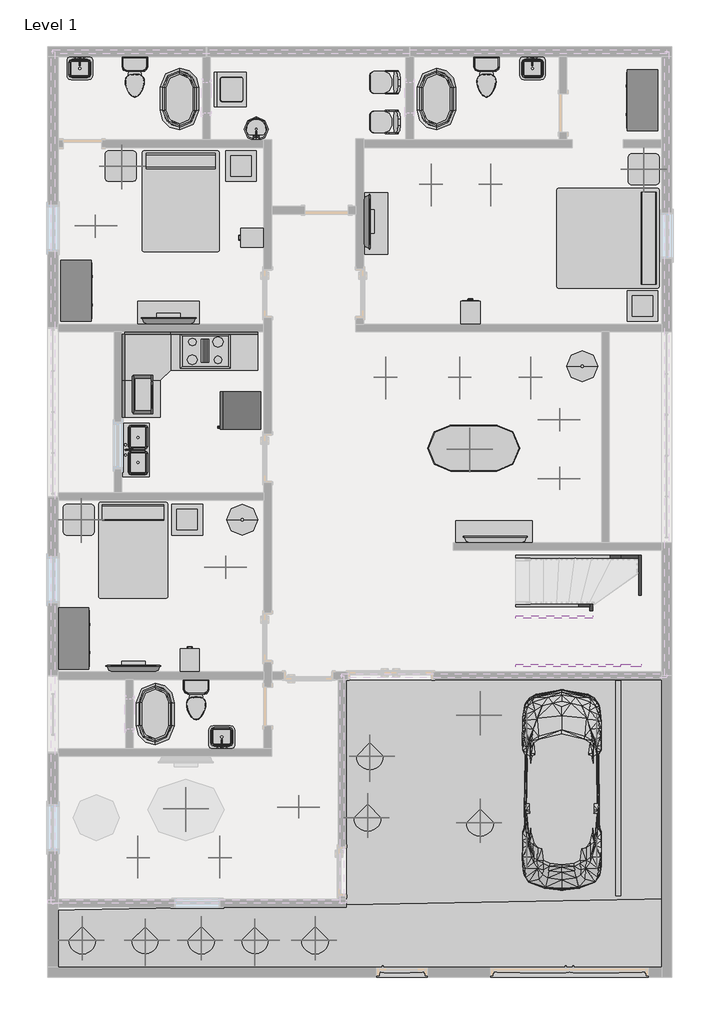
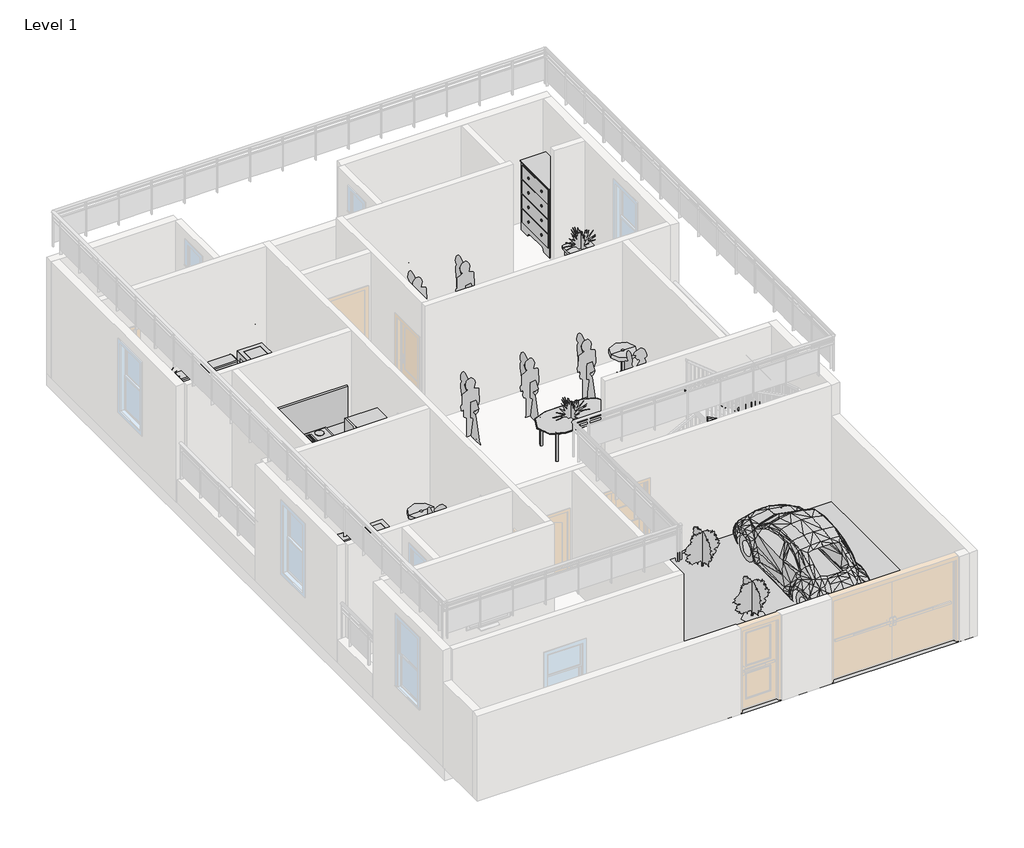
# One storey, part 6 of 6: 28 furniture elements, 20 proxies, 15 flow terminals, 14 geographic elements, 8 members.
"""IFC4 building model written with IfcOpenShell, lengths in millimetres."""

from ifc_helpers import new_model, si_unit, frame, origin, place, context, project, spatial, polyline, outline, extrude, triangles, transform, mapped, element, save
from components import proxy_bb1e6e30, proxy_8a8d5ab2, parking_space_9_x_18_90_deg_fdd9e8f5, rpc_beetle_rpc_beetle_3ce7ba48, rpc_female_69e001fa, proxy_a13a33b2, proxy_718fa39f, flow_terminal_accce45a, flow_terminal_a53be723, flow_terminal_d49f872f, flow_terminal_62a433f7, toilet_domestic_3d_toilet_domestic_3d_f7549cf7, toilet_domestic_3d_toilet_domestic_3d_183bbd19, flow_terminal_04541809, furniture_0253826f, furniture_1fc5af50, furniture_e1791683, furniture_bb55ed6b, furniture_9fa109b2, furniture_3d1d9cbc, furniture_7a3aaa4f, furniture_fdf74506, furniture_b5c51a22, furniture_2c34a4f9, furniture_31d08a24, furniture_c21ab0ed, furniture_87306a90, furniture_1e21b0be, furniture_c625fdf3, rpc_plant_tropical_55f6ff97, rpc_plant_tropical_agave_1_5_93a2a214, rpc_plant_tropical_jungle_flame_3_9c4808c2

model = new_model("IFC4")

# Units and contexts
model_context = context("Model", 3, world=origin())
ifc_project = project(units=[si_unit("LENGTHUNIT", "METRE", prefix="MILLI")], contexts=[model_context])

# Site, building, storey
site = spatial("IfcSite", under=ifc_project)
building = spatial("IfcBuilding", under=site)
storey = spatial("IfcBuildingStorey", under=building, Name="Level 1", Elevation=0.0)

# Proxies
placement = place(None, origin())
element("IfcBuildingElementProxy", 1, Name="Building Element Proxy", at=placement, inside=storey, context=model_context, shape_type="Tessellation", body=[
    triangles([(-14607.1839752, -3299.9680504, 0.0), (-14607.1839752, -4637.9727173, 0.0), (-2211.984169, -4637.9727173, 0.0), (-2211.984169, -3074.4164108, 0.0)], [[1, 2, 3], [3, 4, 1]], closed=False),
])
element("IfcBuildingElementProxy", 2, Name="Building Element Proxy", at=placement, inside=storey, context=model_context, shape_type="Tessellation", body=[
    triangles([(-8688.984169, -3240.9728142, 0.0), (-2211.984169, -3049.3548592, 0.0), (-8841.384169, 1280.2272343, 0.0), (-2211.984169, 1236.1293446, 0.0), (-8638.1843628, 1432.6272343, 0.0), (-2415.1841206, 1280.2272343, 0.0), (-2415.1841206, -3090.3834595, 0.0)], [[3, 1, 5], [5, 1, 7], [7, 2, 4], [4, 6, 7], [7, 6, 5]], closed=False),
])
proxy_shape = proxy_bb1e6e30(model_context)
element("IfcBuildingElementProxy", 3, Name="Cook Top-4 Unit : 36\" x 20\"", ObjectType="Cook Top-4 Unit : 36\" x 20\"", at=placement, inside=storey, context=model_context, shape_type="MappedRepresentation", body=[
    mapped(proxy_shape, transform((-11482.9841185, 7808.0271763, 0.0), x_axis=(1.0, 0.0, 0.0), y_axis=(0.0, 1.0, 0.0), z_axis=(0.0, 0.0, 1.0))),
])
proxy_2_shape = proxy_8a8d5ab2(model_context)
element("IfcBuildingElementProxy", 4, Name="Microwave : 30\" x 16\" x 18\"", ObjectType="Microwave : 30\" x 16\" x 18\"", at=placement, inside=storey, context=model_context, shape_type="MappedRepresentation", body=[
    mapped(proxy_2_shape, transform((-13080.6646243, 6444.1342989, 0.0), x_axis=(0.0, 0.9999999999999999, 0.0), y_axis=(-0.9999999999999999, 0.0, 0.0), z_axis=(0.0, 0.0, 1.0))),
])
parking_space_9_x_18_90_deg_shape = parking_space_9_x_18_90_deg_fdd9e8f5(model_context)
element("IfcBuildingElementProxy", 5, Name="Parking Space : 9' x 18' - 90 deg", ObjectType="Parking Space : 9' x 18' - 90 deg", at=placement, inside=storey, context=model_context, shape_type="MappedRepresentation", body=[
    mapped(parking_space_9_x_18_90_deg_shape, transform((-3278.7841185, -3012.3728237, 0.0), x_axis=(-1.0000000000000004, 0.0, 0.0), y_axis=(0.0, -1.0000000000000004, 0.0), z_axis=(0.0, 0.0, 1.0))),
])
rpc_beetle_rpc_beetle_shape = rpc_beetle_rpc_beetle_3ce7ba48(model_context)
element("IfcBuildingElementProxy", 6, Name="RPC Beetle : RPC Beetle", ObjectType="RPC Beetle : RPC Beetle", at=placement, inside=storey, context=model_context, shape_type="MappedRepresentation", body=[
    mapped(rpc_beetle_rpc_beetle_shape, transform((-4396.3841185, -2148.7728237, 0.0), x_axis=(1.0, 0.0, 0.0), y_axis=(0.0, 1.0, 0.0), z_axis=(0.0, 0.0, 1.0))),
])
rpc_female_shape = rpc_female_69e001fa(model_context)
element("IfcBuildingElementProxy", 7, Name="RPC Female", ObjectType="RPC Female", at=placement, inside=storey, context=model_context, shape_type="MappedRepresentation", body=[
    mapped(rpc_female_shape, transform((-13502.2841185, 10284.5271763, 0.0), x_axis=(0.0, 1.0000000000000002, 0.0), y_axis=(-1.0000000000000002, 0.0, 0.0), z_axis=(0.0, 0.0, 1.0))),
])
element("IfcBuildingElementProxy", 8, Name="RPC Female", ObjectType="RPC Female", at=placement, inside=storey, context=model_context, shape_type="MappedRepresentation", body=[
    mapped(rpc_female_shape, transform((-6996.4115264, 10957.6271763, 0.0), x_axis=(1.0, 0.0, 0.0), y_axis=(0.0, 1.0, 0.0), z_axis=(0.0, 0.0, 1.0))),
])
element("IfcBuildingElementProxy", 9, Name="RPC Female", ObjectType="RPC Female", at=placement, inside=storey, context=model_context, shape_type="MappedRepresentation", body=[
    mapped(rpc_female_shape, transform((-5814.2783903, 10957.6271763, 0.0), x_axis=(1.0, 0.0, 0.0), y_axis=(0.0, 1.0, 0.0), z_axis=(0.0, 0.0, 1.0))),
])
element("IfcBuildingElementProxy", 10, Name="RPC Female", ObjectType="RPC Female", at=placement, inside=storey, context=model_context, shape_type="MappedRepresentation", body=[
    mapped(rpc_female_shape, transform((-6427.2318795, 7122.2271763, 0.0), x_axis=(1.0, 0.0, 0.0), y_axis=(0.0, 1.0, 0.0), z_axis=(0.0, 0.0, 1.0))),
])
element("IfcBuildingElementProxy", 11, Name="RPC Female", ObjectType="RPC Female", at=placement, inside=storey, context=model_context, shape_type="MappedRepresentation", body=[
    mapped(rpc_female_shape, transform((-7900.7506422, 7122.2271763, 0.0), x_axis=(1.0, 0.0, 0.0), y_axis=(0.0, 1.0, 0.0), z_axis=(0.0, 0.0, 1.0))),
])
element("IfcBuildingElementProxy", 12, Name="RPC Female", ObjectType="RPC Female", at=placement, inside=storey, context=model_context, shape_type="MappedRepresentation", body=[
    mapped(rpc_female_shape, transform((-5018.7212974, 7122.2271763, 0.0), x_axis=(1.0, 0.0, 0.0), y_axis=(0.0, 1.0, 0.0), z_axis=(0.0, 0.0, 1.0))),
])
element("IfcBuildingElementProxy", 13, Name="RPC Female", ObjectType="RPC Female", at=placement, inside=storey, context=model_context, shape_type="MappedRepresentation", body=[
    mapped(rpc_female_shape, transform((-4599.5841185, 6441.2059609, 0.0), x_axis=(0.0, -1.0, 0.0), y_axis=(1.0, 0.0, 0.0), z_axis=(0.0, 0.0, 1.0))),
])
element("IfcBuildingElementProxy", 14, Name="RPC Female", ObjectType="RPC Female", at=placement, inside=storey, context=model_context, shape_type="MappedRepresentation", body=[
    mapped(rpc_female_shape, transform((-4599.5841185, 5275.3101398, 0.0), x_axis=(0.0, -1.0, 0.0), y_axis=(1.0, 0.0, 0.0), z_axis=(0.0, 0.0, 1.0))),
])
element("IfcBuildingElementProxy", 15, Name="RPC Female", ObjectType="RPC Female", at=placement, inside=storey, context=model_context, shape_type="MappedRepresentation", body=[
    mapped(rpc_female_shape, transform((-9781.1841185, -1249.3866927, 0.0), x_axis=(0.0, -1.0000000000000004, 0.0), y_axis=(1.0000000000000004, 0.0, 0.0), z_axis=(0.0, 0.0, 1.0))),
])
element("IfcBuildingElementProxy", 16, Name="RPC Female", ObjectType="RPC Female", at=placement, inside=storey, context=model_context, shape_type="MappedRepresentation", body=[
    mapped(rpc_female_shape, transform((-11186.0544122, -2097.9728237, 0.0), x_axis=(-1.0000000000000004, 0.0, 0.0), y_axis=(0.0, -1.0000000000000004, 0.0), z_axis=(0.0, 0.0, 1.0))),
])
element("IfcBuildingElementProxy", 17, Name="RPC Female", ObjectType="RPC Female", at=placement, inside=storey, context=model_context, shape_type="MappedRepresentation", body=[
    mapped(rpc_female_shape, transform((-12811.25893, -2097.9728237, 0.0), x_axis=(-1.0, 0.0, 0.0), y_axis=(0.0, -1.0, 0.0), z_axis=(0.0, 0.0, 1.0))),
])
element("IfcBuildingElementProxy", 18, Name="RPC Female", ObjectType="RPC Female", at=placement, inside=storey, context=model_context, shape_type="MappedRepresentation", body=[
    mapped(rpc_female_shape, transform((-11228.9841185, 3511.6676926, 0.0), x_axis=(0.0, -1.0000000000000004, 0.0), y_axis=(1.0000000000000004, 0.0, 0.0), z_axis=(0.0, 0.0, 1.0))),
])
proxy_3_shape = proxy_a13a33b2(model_context)
element("IfcBuildingElementProxy", 19, Name="Refrigerator : 30\" x 32\" RH", ObjectType="Refrigerator : 30\" x 32\" RH", at=placement, inside=storey, context=model_context, shape_type="MappedRepresentation", body=[
    mapped(proxy_3_shape, transform((-10764.235147, 6622.1646763, 0.0), x_axis=(0.0, -1.0000000000000007, 0.0), y_axis=(1.0000000000000007, 0.0, 0.0), z_axis=(0.0, 0.0, 1.0))),
])
proxy_4_shape = proxy_718fa39f(model_context)
element("IfcBuildingElementProxy", 20, Name="Washer : 27\" x 25\" x 35\"", ObjectType="Washer : 27\" x 25\" x 35\"", at=placement, inside=storey, context=model_context, shape_type="MappedRepresentation", body=[
    mapped(proxy_4_shape, transform((-10708.5345537, 12581.9097078, 0.0), x_axis=(0.0, 1.0000000000000009, 0.0), y_axis=(-1.0000000000000009, 0.0, 0.0), z_axis=(0.0, 0.0, 1.0))),
])

# Flow terminals
flow_terminal_shape = flow_terminal_accce45a(model_context)
element("IfcFlowTerminal", 21, ObjectType="Floor Drain - Round : 5\" Strainer - 2\" Drain", at=placement, inside=storey, context=model_context, shape_type="MappedRepresentation", body=[
    mapped(flow_terminal_shape, transform((-12651.3841185, 12507.0271763, 0.0), x_axis=(1.0, 0.0, 0.0), y_axis=(0.0, 1.0, 0.0), z_axis=(0.0, 0.0, 1.0))),
])
element("IfcFlowTerminal", 22, ObjectType="Floor Drain - Round : 5\" Strainer - 2\" Drain", at=placement, inside=storey, context=model_context, shape_type="MappedRepresentation", body=[
    mapped(flow_terminal_shape, transform((-6275.9841185, 12303.8271763, 0.0), x_axis=(1.0, 0.0, 0.0), y_axis=(0.0, 1.0, 0.0), z_axis=(0.0, 0.0, 1.0))),
])
element("IfcFlowTerminal", 23, ObjectType="Floor Drain - Round : 5\" Strainer - 2\" Drain", at=placement, inside=storey, context=model_context, shape_type="MappedRepresentation", body=[
    mapped(flow_terminal_shape, transform((-10466.9841185, 13446.8271763, 0.0), x_axis=(1.0, 0.0, 0.0), y_axis=(0.0, 1.0, 0.0), z_axis=(0.0, 0.0, 1.0))),
])
element("IfcFlowTerminal", 24, ObjectType="Floor Drain - Round : 5\" Strainer - 2\" Drain", at=placement, inside=storey, context=model_context, shape_type="MappedRepresentation", body=[
    mapped(flow_terminal_shape, transform((-11965.5841185, 86.4271763, 0.0), x_axis=(1.0, 0.0, 0.0), y_axis=(0.0, 1.0, 0.0), z_axis=(0.0, 0.0, 1.0))),
])
flow_terminal_2_shape = flow_terminal_a53be723(model_context)
element("IfcFlowTerminal", 25, ObjectType="Sink Kitchen-Double : 42\" x 21\"", at=placement, inside=storey, context=model_context, shape_type="MappedRepresentation", body=[
    mapped(flow_terminal_2_shape, transform((-12852.2387174, 5823.8379357, 0.0), x_axis=(0.0, 1.0000000000000002, 0.0), y_axis=(-1.0000000000000002, 0.0, 0.0), z_axis=(0.0, 0.0, 1.0))),
])
flow_terminal_3_shape = flow_terminal_d49f872f(model_context)
element("IfcFlowTerminal", 26, ObjectType="Sink Vanity-Round : 19\" x 19\"", at=placement, inside=storey, context=model_context, shape_type="MappedRepresentation", body=[
    mapped(flow_terminal_3_shape, transform((-10370.3323779, 12298.7524416, 0.0), x_axis=(-1.0000000000000004, 0.0, 0.0), y_axis=(0.0, -1.0000000000000004, 0.0), z_axis=(0.0, 0.0, 1.0))),
])
flow_terminal_4_shape = flow_terminal_62a433f7(model_context)
element("IfcFlowTerminal", 27, ObjectType="Sink Vanity-Square : 20\" x 18\"", at=placement, inside=storey, context=model_context, shape_type="MappedRepresentation", body=[
    mapped(flow_terminal_4_shape, transform((-13987.8733591, 13469.8817752, 0.0), x_axis=(1.0, 0.0, 0.0), y_axis=(0.0, 1.0, 0.0), z_axis=(0.0, 0.0, 1.0))),
])
element("IfcFlowTerminal", 28, ObjectType="Sink Vanity-Square : 20\" x 18\"", at=placement, inside=storey, context=model_context, shape_type="MappedRepresentation", body=[
    mapped(flow_terminal_4_shape, transform((-4996.2733591, 13469.8817752, 0.0), x_axis=(1.0, 0.0, 0.0), y_axis=(0.0, 1.0, 0.0), z_axis=(0.0, 0.0, 1.0))),
])
element("IfcFlowTerminal", 29, ObjectType="Sink Vanity-Square : 20\" x 18\"", at=placement, inside=storey, context=model_context, shape_type="MappedRepresentation", body=[
    mapped(flow_terminal_4_shape, transform((-11137.0948779, 88.7725774, 0.0), x_axis=(-1.0000000000000004, 0.0, 0.0), y_axis=(0.0, -1.0000000000000004, 0.0), z_axis=(0.0, 0.0, 1.0))),
])
toilet_domestic_3d_toilet_domestic_3d_shape = toilet_domestic_3d_toilet_domestic_3d_f7549cf7(model_context)
toilet_domestic_3d_toilet_domestic_3d_2_shape = toilet_domestic_3d_toilet_domestic_3d_183bbd19(model_context)
element("IfcFlowTerminal", 30, ObjectType="Toilet-Domestic-3D : Toilet-Domestic-3D", at=placement, inside=storey, context=model_context, shape_type="MappedRepresentation", body=[
    mapped(toilet_domestic_3d_toilet_domestic_3d_shape, transform((-5894.9841185, 13155.3311489, 0.0), x_axis=(1.0, 0.0, 0.0), y_axis=(0.0, 1.0, 0.0), z_axis=(0.0, 0.0, 1.0))),
    mapped(toilet_domestic_3d_toilet_domestic_3d_2_shape, transform((-5894.9841185, 13155.3311489, 0.0), x_axis=(1.0, 0.0, 0.0), y_axis=(0.0, 1.0, 0.0), z_axis=(0.0, 0.0, 1.0))),
])
element("IfcFlowTerminal", 31, ObjectType="Toilet-Domestic-3D : Toilet-Domestic-3D", at=placement, inside=storey, context=model_context, shape_type="MappedRepresentation", body=[
    mapped(toilet_domestic_3d_toilet_domestic_3d_shape, transform((-12879.9841185, 13155.3311489, 0.0), x_axis=(1.0, 0.0, 0.0), y_axis=(0.0, 1.0, 0.0), z_axis=(0.0, 0.0, 1.0))),
    mapped(toilet_domestic_3d_toilet_domestic_3d_2_shape, transform((-12879.9841185, 13155.3311489, 0.0), x_axis=(1.0, 0.0, 0.0), y_axis=(0.0, 1.0, 0.0), z_axis=(0.0, 0.0, 1.0))),
])
element("IfcFlowTerminal", 32, ObjectType="Toilet-Domestic-3D : Toilet-Domestic-3D", at=placement, inside=storey, context=model_context, shape_type="MappedRepresentation", body=[
    mapped(toilet_domestic_3d_toilet_domestic_3d_shape, transform((-11660.7841185, 785.5311489, 0.0), x_axis=(1.0, 0.0, 0.0), y_axis=(0.0, 1.0, 0.0), z_axis=(0.0, 0.0, 1.0))),
    mapped(toilet_domestic_3d_toilet_domestic_3d_2_shape, transform((-11660.7841185, 785.5311489, 0.0), x_axis=(1.0, 0.0, 0.0), y_axis=(0.0, 1.0, 0.0), z_axis=(0.0, 0.0, 1.0))),
])
flow_terminal_5_shape = flow_terminal_04541809(model_context)
element("IfcFlowTerminal", 33, ObjectType="Tub-Free Standing-3D : 30\" x 60\"", at=placement, inside=storey, context=model_context, shape_type="MappedRepresentation", body=[
    mapped(flow_terminal_5_shape, transform((-11990.9841185, 12811.8271763, 0.0), x_axis=(-1.0, 0.0, 0.0), y_axis=(0.0, -1.0, 0.0), z_axis=(0.0, 0.0, 1.0))),
])
element("IfcFlowTerminal", 34, ObjectType="Tub-Free Standing-3D : 30\" x 60\"", at=placement, inside=storey, context=model_context, shape_type="MappedRepresentation", body=[
    mapped(flow_terminal_5_shape, transform((-6885.5841185, 12811.8271763, 0.0), x_axis=(-1.0, 0.0, 0.0), y_axis=(0.0, -1.0, 0.0), z_axis=(0.0, 0.0, 1.0))),
])
element("IfcFlowTerminal", 35, ObjectType="Tub-Free Standing-3D : 30\" x 60\"", at=placement, inside=storey, context=model_context, shape_type="MappedRepresentation", body=[
    mapped(flow_terminal_5_shape, transform((-12473.5841185, 594.4271763, 0.0), x_axis=(1.0000000000000007, 0.0, 0.0), y_axis=(0.0, 1.0000000000000007, 0.0), z_axis=(0.0, 0.0, 1.0))),
])

# Furniture
furniture_shape = furniture_0253826f(model_context)
element("IfcFurniture", 36, ObjectType="Bed-Standard.0001 : Double 54\" x 75\"", at=placement, inside=storey, context=model_context, shape_type="MappedRepresentation", body=[
    mapped(furniture_shape, transform((-13183.2226431, 3891.2222582, 0.0), x_axis=(1.0, 0.0, 0.0), y_axis=(0.0, 1.0, 0.0), z_axis=(0.0, 0.0, 1.0))),
])
furniture_2_shape = furniture_1fc5af50(model_context)
element("IfcFurniture", 37, ObjectType="Bed-Standard.0001 : King 78\" x 80\"", at=placement, inside=storey, context=model_context, shape_type="MappedRepresentation", body=[
    mapped(furniture_2_shape, transform((-3436.3890365, 10314.7157009, 0.0), x_axis=(0.0, -0.9999999999999998, 0.0), y_axis=(0.9999999999999998, 0.0, 0.0), z_axis=(0.0, 0.0, 1.0))),
])
furniture_3_shape = furniture_e1791683(model_context)
element("IfcFurniture", 38, ObjectType="Bed-Standard.0001 : Queen 60\" x 79\"", at=placement, inside=storey, context=model_context, shape_type="MappedRepresentation", body=[
    mapped(furniture_3_shape, transform((-12237.0726431, 10825.4222582, 0.0), x_axis=(1.0, 0.0, 0.0), y_axis=(0.0, 1.0, 0.0), z_axis=(0.0, 0.0, 1.0))),
])
furniture_4_shape = furniture_bb55ed6b(model_context)
element("IfcFurniture", 39, ObjectType="Cabinet-File 2 Drawer : 15\" x 18\"", at=placement, inside=storey, context=model_context, shape_type="MappedRepresentation", body=[
    mapped(furniture_4_shape, transform((-10401.0498184, 9928.0307292, 0.0), x_axis=(0.0, -1.0000000000000002, 0.0), y_axis=(1.0000000000000002, 0.0, 0.0), z_axis=(0.0, 0.0, 1.0))),
])
element("IfcFurniture", 40, ObjectType="Cabinet-File 2 Drawer : 15\" x 18\"", at=placement, inside=storey, context=model_context, shape_type="MappedRepresentation", body=[
    mapped(furniture_4_shape, transform((-6340.3805655, 8427.8928761, 0.0), x_axis=(-0.9999999999999998, 0.0, 0.0), y_axis=(0.0, -0.9999999999999998, 0.0), z_axis=(0.0, 0.0, 1.0))),
])
element("IfcFurniture", 41, ObjectType="Cabinet-File 2 Drawer : 15\" x 18\"", at=placement, inside=storey, context=model_context, shape_type="MappedRepresentation", body=[
    mapped(furniture_4_shape, transform((-11915.6805655, 1519.0928761, 0.0), x_axis=(-1.0000000000000002, 0.0, 0.0), y_axis=(0.0, -1.0000000000000002, 0.0), z_axis=(0.0, 0.0, 1.0))),
])
furniture_5_shape = furniture_9fa109b2(model_context)
element("IfcFurniture", 42, ObjectType="Dresser : 48\" x 72\" x 24\"", at=placement, inside=storey, context=model_context, shape_type="MappedRepresentation", body=[
    mapped(furniture_5_shape, transform((-2433.0211644, 12517.2339164, 0.0), x_axis=(0.0, -1.0000000000000007, 0.0), y_axis=(1.0000000000000007, 0.0, 0.0), z_axis=(0.0, 0.0, 1.0))),
])
element("IfcFurniture", 43, ObjectType="Dresser : 48\" x 72\" x 24\"", at=placement, inside=storey, context=model_context, shape_type="MappedRepresentation", body=[
    mapped(furniture_5_shape, transform((-14411.5470726, 9271.0204361, 0.0), x_axis=(0.0, 1.0, 0.0), y_axis=(-1.0, 0.0, 0.0), z_axis=(0.0, 0.0, 1.0))),
])
element("IfcFurniture", 44, ObjectType="Dresser : 48\" x 72\" x 24\"", at=placement, inside=storey, context=model_context, shape_type="MappedRepresentation", body=[
    mapped(furniture_5_shape, transform((-14462.3470726, 2362.2204361, 0.0), x_axis=(0.0, 1.0000000000000002, 0.0), y_axis=(-1.0000000000000002, 0.0, 0.0), z_axis=(0.0, 0.0, 1.0))),
])
furniture_6_shape = furniture_3d1d9cbc(model_context)
element("IfcFurniture", 45, ObjectType="Seating-Auditorium : 18\" x 24\" x 30\"", at=placement, inside=storey, context=model_context, shape_type="MappedRepresentation", body=[
    mapped(furniture_6_shape, transform((-7711.7087087, 12981.2993074, 0.0), x_axis=(0.0, 1.0000000000000002, 0.0), y_axis=(-1.0000000000000002, 0.0, 0.0), z_axis=(0.0, 0.0, 1.0))),
])
element("IfcFurniture", 46, ObjectType="Seating-Auditorium : 18\" x 24\" x 30\"", at=placement, inside=storey, context=model_context, shape_type="MappedRepresentation", body=[
    mapped(furniture_6_shape, transform((-7711.7087087, 12193.8993074, 0.0), x_axis=(0.0, 1.0000000000000002, 0.0), y_axis=(-1.0000000000000002, 0.0, 0.0), z_axis=(0.0, 0.0, 1.0))),
])
furniture_7_shape = furniture_7a3aaa4f(model_context)
element("IfcFurniture", 47, ObjectType="TV - Flat Screen : 42\"", at=placement, inside=storey, context=model_context, shape_type="MappedRepresentation", body=[
    mapped(furniture_7_shape, transform((-12210.8286326, 8399.9657999, 1041.4), x_axis=(-1.0000000000000004, 0.0, 0.0), y_axis=(0.0, -1.0000000000000004, 0.0), z_axis=(0.0, 0.0, 1.0))),
])
element("IfcFurniture", 48, ObjectType="TV - Flat Screen : 42\"", at=placement, inside=storey, context=model_context, shape_type="MappedRepresentation", body=[
    mapped(furniture_7_shape, transform((-8274.8454949, 10377.3716904, 1041.4), x_axis=(0.0, 1.0000000000000002, 0.0), y_axis=(-1.0000000000000002, 0.0, 0.0), z_axis=(0.0, 0.0, 1.0))),
])
element("IfcFurniture", 49, ObjectType="TV - Flat Screen : 42\"", at=placement, inside=storey, context=model_context, shape_type="MappedRepresentation", body=[
    mapped(furniture_7_shape, transform((-12909.3286326, 1491.1657999, 1041.4), x_axis=(-1.0, 0.0, 0.0), y_axis=(0.0, -1.0, 0.0), z_axis=(0.0, 0.0, 1.0))),
])
furniture_8_shape = furniture_fdf74506(model_context)
element("IfcFurniture", 50, ObjectType="TV - Flat Screen : 50\"", at=placement, inside=storey, context=model_context, shape_type="MappedRepresentation", body=[
    mapped(furniture_8_shape, transform((-5721.1286326, 4056.5657999, 0.0), x_axis=(-1.0000000000000004, 0.0, 0.0), y_axis=(0.0, -1.0000000000000004, 0.0), z_axis=(0.0, 0.0, 1.0))),
])
furniture_9_shape = furniture_b5c51a22(model_context)
element("IfcFurniture", 51, ObjectType="Table-Coffee : 24\" x 24\" x 24\"", at=placement, inside=storey, context=model_context, shape_type="MappedRepresentation", body=[
    mapped(furniture_9_shape, transform((-10790.0498852, 11383.1160985, 0.0), x_axis=(1.0, 0.0, 0.0), y_axis=(0.0, 1.0, 0.0), z_axis=(0.0, 0.0, 1.0))),
])
element("IfcFurniture", 52, ObjectType="Table-Coffee : 24\" x 24\" x 24\"", at=placement, inside=storey, context=model_context, shape_type="MappedRepresentation", body=[
    mapped(furniture_9_shape, transform((-2814.4498852, 8601.8160985, 0.0), x_axis=(1.0, 0.0, 0.0), y_axis=(0.0, 1.0, 0.0), z_axis=(0.0, 0.0, 1.0))),
])
element("IfcFurniture", 53, ObjectType="Table-Coffee : 24\" x 24\" x 24\"", at=placement, inside=storey, context=model_context, shape_type="MappedRepresentation", body=[
    mapped(furniture_9_shape, transform((-11856.8498852, 4360.0160985, 0.0), x_axis=(1.0, 0.0, 0.0), y_axis=(0.0, 1.0, 0.0), z_axis=(0.0, 0.0, 1.0))),
])
furniture_10_shape = furniture_2c34a4f9(model_context)
element("IfcFurniture", 54, ObjectType="Table-Dining Oval : 36\" x 72\"", at=placement, inside=storey, context=model_context, shape_type="MappedRepresentation", body=[
    mapped(furniture_10_shape, transform((-5747.1644464, 6235.7255369, 0.0), x_axis=(1.0, 0.0, 0.0), y_axis=(0.0, 1.0, 0.0), z_axis=(0.0, 0.0, 1.0))),
])
furniture_11_shape = furniture_31d08a24(model_context)
element("IfcFurniture", 55, ObjectType="Table-End : 24\" x 24\"", at=placement, inside=storey, context=model_context, shape_type="MappedRepresentation", body=[
    mapped(furniture_11_shape, transform((-13467.9177488, 11325.9271763, 0.0), x_axis=(1.0, 0.0, 0.0), y_axis=(0.0, 1.0, 0.0), z_axis=(0.0, 0.0, 1.0))),
])
element("IfcFurniture", 56, ObjectType="Table-End : 24\" x 24\"", at=placement, inside=storey, context=model_context, shape_type="MappedRepresentation", body=[
    mapped(furniture_11_shape, transform((-3079.3177488, 11262.4271763, 0.0), x_axis=(1.0, 0.0, 0.0), y_axis=(0.0, 1.0, 0.0), z_axis=(0.0, 0.0, 1.0))),
])
element("IfcFurniture", 57, ObjectType="Table-End : 24\" x 24\"", at=placement, inside=storey, context=model_context, shape_type="MappedRepresentation", body=[
    mapped(furniture_11_shape, transform((-14299.7677488, 4302.8271763, 0.0), x_axis=(1.0, 0.0, 0.0), y_axis=(0.0, 1.0, 0.0), z_axis=(0.0, 0.0, 1.0))),
])
furniture_12_shape = furniture_c21ab0ed(model_context)
element("IfcFurniture", 58, ObjectType="Table-Rectangular : 72\" x 30\"", at=placement, inside=storey, context=model_context, shape_type="MappedRepresentation", body=[
    mapped(furniture_12_shape, transform((-8079.3841185, 10335.3271763, 0.0), x_axis=(0.0, 1.0000000000000002, 0.0), y_axis=(-1.0000000000000002, 0.0, 0.0), z_axis=(0.0, 0.0, 1.0))),
])
element("IfcFurniture", 59, ObjectType="Table-Rectangular : 72\" x 30\"", at=placement, inside=storey, context=model_context, shape_type="MappedRepresentation", body=[
    mapped(furniture_12_shape, transform((-12206.8841185, 8570.0271763, 0.0), x_axis=(1.0, 0.0, 0.0), y_axis=(0.0, 1.0, 0.0), z_axis=(0.0, 0.0, 1.0))),
])
furniture_13_shape = furniture_87306a90(model_context)
element("IfcFurniture", 60, ObjectType="Table-Rectangular : 72\" x 30\" 2", at=placement, inside=storey, context=model_context, shape_type="MappedRepresentation", body=[
    mapped(furniture_13_shape, transform((-5742.5841185, 4208.0271763, 0.0), x_axis=(1.0, 0.0, 0.0), y_axis=(0.0, 1.0, 0.0), z_axis=(0.0, 0.0, 1.0))),
])
furniture_14_shape = furniture_1e21b0be(model_context)
element("IfcFurniture", 61, ObjectType="Table-Round : 36\" Diameter", at=placement, inside=storey, context=model_context, shape_type="MappedRepresentation", body=[
    mapped(furniture_14_shape, transform((-3989.9841185, 7503.2271763, 0.0), x_axis=(1.0, 0.0, 0.0), y_axis=(0.0, 1.0, 0.0), z_axis=(0.0, 0.0, 1.0))),
])
element("IfcFurniture", 62, ObjectType="Table-Round : 36\" Diameter", at=placement, inside=storey, context=model_context, shape_type="MappedRepresentation", body=[
    mapped(furniture_14_shape, transform((-10746.3841185, 4455.2271763, 0.0), x_axis=(1.0, 0.0, 0.0), y_axis=(0.0, 1.0, 0.0), z_axis=(0.0, 0.0, 1.0))),
])
furniture_15_shape = furniture_c625fdf3(model_context)
element("IfcFurniture", 63, ObjectType="Work Station Cubicle : 96\" x 96\"", at=placement, inside=storey, context=model_context, shape_type="MappedRepresentation", body=[
    mapped(furniture_15_shape, transform((-13002.2523663, 8684.0501839, 0.0), x_axis=(1.0, 0.0, 0.0), y_axis=(0.0, 1.0, 0.0), z_axis=(0.0, 0.0, 1.0))),
])

# Geographic elements
rpc_plant_tropical_shape = rpc_plant_tropical_55f6ff97(model_context)
element("IfcGeographicElement", 64, ObjectType="RPC Plant - Tropical", at=placement, inside=storey, context=model_context, shape_type="MappedRepresentation", body=[
    mapped(rpc_plant_tropical_shape, transform((-12676.7841185, -3901.3728237, 0.0), x_axis=(1.0, 0.0, 0.0), y_axis=(0.0, 1.0, 0.0), z_axis=(0.0, 0.0, 1.0))),
])
element("IfcGeographicElement", 65, ObjectType="RPC Plant - Tropical", at=placement, inside=storey, context=model_context, shape_type="MappedRepresentation", body=[
    mapped(rpc_plant_tropical_shape, transform((-10492.3841185, -3901.3728237, 0.0), x_axis=(1.0, 0.0, 0.0), y_axis=(0.0, 1.0, 0.0), z_axis=(0.0, 0.0, 1.0))),
])
element("IfcGeographicElement", 66, ObjectType="RPC Plant - Tropical", at=placement, inside=storey, context=model_context, shape_type="MappedRepresentation", body=[
    mapped(rpc_plant_tropical_shape, transform((-8210.1158104, -243.7728237, 0.0), x_axis=(1.0, 0.0, 0.0), y_axis=(0.0, 1.0, 0.0), z_axis=(0.0, 0.0, 1.0))),
])
rpc_plant_tropical_agave_1_5_shape = rpc_plant_tropical_agave_1_5_93a2a214(model_context)
element("IfcGeographicElement", 67, ObjectType="RPC Plant - Tropical : Agave - 1.5'", at=placement, inside=storey, context=model_context, shape_type="MappedRepresentation", body=[
    mapped(rpc_plant_tropical_agave_1_5_shape, transform((-13133.9841185, 11478.3271763, 609.6), x_axis=(1.0, 0.0, 0.0), y_axis=(0.0, 1.0, 0.0), z_axis=(0.0, 0.0, 1.0))),
])
element("IfcGeographicElement", 68, ObjectType="RPC Plant - Tropical : Agave - 1.5'", at=placement, inside=storey, context=model_context, shape_type="MappedRepresentation", body=[
    mapped(rpc_plant_tropical_agave_1_5_shape, transform((-2770.7841185, 11414.8271763, 609.6), x_axis=(1.0, 0.0, 0.0), y_axis=(0.0, 1.0, 0.0), z_axis=(0.0, 0.0, 1.0))),
])
element("IfcGeographicElement", 69, ObjectType="RPC Plant - Tropical : Agave - 1.5'", at=placement, inside=storey, context=model_context, shape_type="MappedRepresentation", body=[
    mapped(rpc_plant_tropical_agave_1_5_shape, transform((-6225.1841185, 5852.2271763, 736.6), x_axis=(1.0, 0.0, 0.0), y_axis=(0.0, 1.0, 0.0), z_axis=(0.0, 0.0, 1.0))),
])
element("IfcGeographicElement", 70, ObjectType="RPC Plant - Tropical : Agave - 1.5'", at=placement, inside=storey, context=model_context, shape_type="MappedRepresentation", body=[
    mapped(rpc_plant_tropical_agave_1_5_shape, transform((-13940.4341185, 4455.2271763, 609.6), x_axis=(1.0, 0.0, 0.0), y_axis=(0.0, 1.0, 0.0), z_axis=(0.0, 0.0, 1.0))),
])
element("IfcGeographicElement", 71, ObjectType="RPC Plant - Tropical : Agave - 1.5'", at=placement, inside=storey, context=model_context, shape_type="MappedRepresentation", body=[
    mapped(rpc_plant_tropical_agave_1_5_shape, transform((-11863.9841185, -1285.1728237, 736.6), x_axis=(1.0, 0.0, 0.0), y_axis=(0.0, 1.0, 0.0), z_axis=(0.0, 0.0, 1.0))),
])
rpc_plant_tropical_jungle_flame_3_shape = rpc_plant_tropical_jungle_flame_3_9c4808c2(model_context)
element("IfcGeographicElement", 72, ObjectType="RPC Plant - Tropical : Jungle Flame - 3'", at=placement, inside=storey, context=model_context, shape_type="MappedRepresentation", body=[
    mapped(rpc_plant_tropical_jungle_flame_3_shape, transform((-13921.3841185, -3901.3728237, 0.0), x_axis=(1.0, 0.0, 0.0), y_axis=(0.0, 1.0, 0.0), z_axis=(0.0, 0.0, 1.0))),
])
element("IfcGeographicElement", 73, ObjectType="RPC Plant - Tropical : Jungle Flame - 3'", at=placement, inside=storey, context=model_context, shape_type="MappedRepresentation", body=[
    mapped(rpc_plant_tropical_jungle_flame_3_shape, transform((-9298.5841185, -3901.3728237, 0.0), x_axis=(1.0, 0.0, 0.0), y_axis=(0.0, 1.0, 0.0), z_axis=(0.0, 0.0, 1.0))),
])
element("IfcGeographicElement", 74, ObjectType="RPC Plant - Tropical : Jungle Flame - 3'", at=placement, inside=storey, context=model_context, shape_type="MappedRepresentation", body=[
    mapped(rpc_plant_tropical_jungle_flame_3_shape, transform((-11559.1841185, -3901.3728237, 0.0), x_axis=(1.0, 0.0, 0.0), y_axis=(0.0, 1.0, 0.0), z_axis=(0.0, 0.0, 1.0))),
])
element("IfcGeographicElement", 75, ObjectType="RPC Plant - Tropical : Jungle Flame - 3'", at=placement, inside=storey, context=model_context, shape_type="MappedRepresentation", body=[
    mapped(rpc_plant_tropical_jungle_flame_3_shape, transform((-6021.9841185, 569.0271763, 0.0), x_axis=(1.0, 0.0, 0.0), y_axis=(0.0, 1.0, 0.0), z_axis=(0.0, 0.0, 1.0))),
])
element("IfcGeographicElement", 76, ObjectType="RPC Plant - Tropical : Jungle Flame - 3'", at=placement, inside=storey, context=model_context, shape_type="MappedRepresentation", body=[
    mapped(rpc_plant_tropical_jungle_flame_3_shape, transform((-6021.9841185, -1564.5728237, 0.0), x_axis=(1.0, 0.0, 0.0), y_axis=(0.0, 1.0, 0.0), z_axis=(0.0, 0.0, 1.0))),
])
element("IfcGeographicElement", 77, ObjectType="RPC Plant - Tropical : Jungle Flame - 3'", at=placement, inside=storey, context=model_context, shape_type="MappedRepresentation", body=[
    mapped(rpc_plant_tropical_jungle_flame_3_shape, transform((-8257.1841185, -1462.9728237, 0.0), x_axis=(1.0, 0.0, 0.0), y_axis=(0.0, 1.0, 0.0), z_axis=(0.0, 0.0, 1.0))),
])

# Members
element("IfcMember", 78, ObjectType="Stringer - 2\" Width", at=placement, inside=storey, context=model_context, shape_type="SweptSolid", body=[
    extrude(outline(polyline([(229.639954, -5314.5158104), (0.0, -5314.5158104), (0.0, -5094.7534928), (962.500629, -3227.0986187), (1305.3956453, -3227.0986187), (229.639954, -5314.5158104)])), frame((0.0, 3693.2271763, 0.0), z_axis=(0.0, 1.0, 0.0), x_axis=(0.0, 0.0, 1.0)), (0.0, 0.0, 1.0), 50.8),
])
element("IfcMember", 79, ObjectType="Stringer - 2\" Width", at=placement, inside=storey, context=model_context, shape_type="SweptSolid", body=[
    extrude(outline(polyline([(-3227.0986187, 3693.2271763), (-3227.0986187, 3744.0271763), (-2872.3841185, 3744.0271763), (-2872.3841185, 3693.2271763), (-3227.0986187, 3693.2271763)])), frame((0.0, 0.0, 962.500629), z_axis=(0.0, 0.0, 1.0), x_axis=(1.0, 0.0, 0.0)), (0.0, 0.0, 1.0), 342.8950162),
])
element("IfcMember", 80, ObjectType="Stringer - 2\" Width", at=placement, inside=storey, context=model_context, shape_type="SweptSolid", body=[
    extrude(outline(polyline([(3744.0271763, 1289.0952212), (3744.0271763, 1000.5956453), (3574.5046933, 1000.5956453), (1585.0271763, 1638.9682298), (1585.0271763, 1969.9972697), (1622.0072936, 1969.9972697), (3744.0271763, 1289.0952212)])), frame((-2872.3841185, 0.0, 0.0), z_axis=(1.0, 0.0, 0.0), x_axis=(0.0, 1.0, 0.0)), (0.0, 0.0, 1.0), 50.8),
])
element("IfcMember", 81, ObjectType="Stringer - 2\" Width", at=placement, inside=storey, context=model_context, shape_type="SweptSolid", body=[
    extrude(outline(polyline([(-2821.5841185, 1585.0271763), (-2821.5841185, 1534.2271763), (-3227.0986187, 1534.2271763), (-3227.0986187, 1585.0271763), (-2821.5841185, 1585.0271763)])), frame((0.0, 0.0, 1649.8904473), z_axis=(0.0, 0.0, 1.0), x_axis=(1.0, 0.0, 0.0)), (0.0, 0.0, 1.0), 320.1068224),
])
element("IfcMember", 82, ObjectType="Stringer - 2\" Width", at=placement, inside=storey, context=model_context, shape_type="SweptSolid", body=[
    extrude(outline(polyline([(1649.8904473, -3227.0986187), (1969.9972697, -3227.0986187), (3045.7529609, -5314.5158104), (2725.6461385, -5314.5158104), (1649.8904473, -3227.0986187)])), frame((0.0, 1534.2271763, 0.0), z_axis=(0.0, 1.0, 0.0), x_axis=(0.0, 0.0, 1.0)), (0.0, 0.0, 1.0), 50.8),
])
element("IfcMember", 83, ObjectType="Stringer - 2\" Width", at=placement, inside=storey, context=model_context, shape_type="SweptSolid", body=[
    extrude(outline(polyline([(176.1764461, -5314.5158104), (0.0, -5314.5158104), (0.0, -5048.2541658), (987.1410923, -3837.5841185), (1380.418648, -3837.5841185), (176.1764461, -5314.5158104)])), frame((0.0, 2728.0271763, 0.0), z_axis=(0.0, 1.0, 0.0), x_axis=(0.0, 0.0, 1.0)), (0.0, 0.0, 1.0), 50.8),
])
element("IfcMember", 84, ObjectType="Stringer - 2\" Width", at=placement, inside=storey, context=model_context, shape_type="SweptSolid", body=[
    extrude(outline(polyline([(2778.8271763, 1573.2682978), (2778.8271763, 1028.5617647), (2744.5849589, 1028.5617647), (2550.2271763, 1360.465107), (2550.2271763, 1926.1409689), (2572.1900588, 1926.1409689), (2778.8271763, 1573.2682978)])), frame((-3837.5841185, 0.0, 0.0), z_axis=(1.0, 0.0, 0.0), x_axis=(0.0, 1.0, 0.0)), (0.0, 0.0, 1.0), 50.8),
])
element("IfcMember", 85, ObjectType="Stringer - 2\" Width", at=placement, inside=storey, context=model_context, shape_type="SweptSolid", body=[
    extrude(outline(polyline([(1532.8634131, -3786.7841185), (1926.1409689, -3786.7841185), (3171.8038432, -5314.5158104), (2778.5262875, -5314.5158104), (1532.8634131, -3786.7841185)])), frame((0.0, 2499.4271763, 0.0), z_axis=(0.0, 1.0, 0.0), x_axis=(0.0, 0.0, 1.0)), (0.0, 0.0, 1.0), 50.8),
])

save(model, "model.ifc")

# Revit data of these elements
# Type "Cook Top-4 Unit : 36\" x 20\""
#   Assembly Code = "E1090400"
#   Depth = 2' - 0"
#   Width = 3' - 0"
#   Burner Material = Steel, Chrome Plated
#   Cooktop Material = Steel, Polished
#   Default Elevation = 0
# Type "Microwave : 30\" x 16\" x 18\""
#   Assembly Code = "E1090400"
#   Depth = 1' - 4"
#   Height = 1' - 6"
#   Width = 2' - 6"
#   Microwave Material = Laminate, Linen, Matte
#   Default Elevation = 0
# Type "Parking Space : 9' x 18' - 90 deg"
#   Angle = 90.00°
#   Parking Length = 18' - 0"
#   Parking Width = 9' - 0"
#   pl = 14' - 0"
#   pw = 7' - 0"
# Type "RPC Beetle : RPC Beetle"
#   built-in parameter 1005195 = "RPC-16-0U6E-L4EG-ENH1-J3KF-SVEL-0TX4-C0"
#   Height = 0
# Type "RPC Female"
#   built-in parameter 1005195 = "RPC-8-FXA2-QQQ0-UGV2-6"
#   Height = 0
# Type "Refrigerator : 30\" x 32\" RH"
#   Label = "REF."
#   Assembly Code = "E1090400"
#   Depth = 2' - 7 3/4"
#   Handle = 2' - 3"
#   Height = 5' - 10"
#   Rear Clearance = 0' - 2"
#   Top Door Height = 1' - 8"
#   Width = 2' - 5 3/8"
#   Material = Carpet (1)
#   Default Elevation = 0
# Type "Washer : 27\" x 25\" x 35\""
#   Label = "W"
#   Assembly Code = "E1090400"
#   Depth = 2' - 1"
#   Height = 2' - 11"
#   Width = 2' - 3"
#   Washer Material = Steel, Paint Finish, Ivory, Matte
#   Default Elevation = 0
# Type "Floor Drain - Round : 5\" Strainer - 2\" Drain"
#   WFU = 2
#   Strainer Height = 0' - 3 1/4"
#   Strainer Radius = 0' - 2 1/2"
#   Strainer Diameter = 0' - 5"
#   Radius 6 = 0' - 0 5/8"
#   Radius 5 = 0' - 1 1/4"
#   Radius 4 = 0' - 1 7/8"
#   Radius 2 = 0' - 3.04167"
#   Radius 1 = 0' - 2.02083"
#   Radius 3 = 0' - 2 1/32"
#   Pipe Radius = 1"
#   Pipe Diameter = 2"
#   Height 2 = 0' - 0.725"
#   Height 1 = 0' - 1 13/16"
#   Body Radius = 0' - 4 1/16"
#   Body Height = 0' - 3 5/8"
#   Body Diameter = 0' - 8 1/8"
#   Drain Material = none
#   HWFU = 0
#   Default Elevation = 0
#   CWFU = 0
# Type "Sink Kitchen-Double : 42\" x 21\""
#   Assembly Code = "D2010410"
#   Counter Height = 3' - 0"
#   Depth = 1' - 9"
#   Width = 3' - 6"
#   Faucet Material = Steel, Polished
#   Sink Material = Steel, Polished
#   Default Elevation = 0
# Type "Sink Vanity-Round : 19\" x 19\""
#   Assembly Code = "D2010400"
#   Top Of Counter = 2' - 7"
#   Basin Material = Porcelain, Linen
#   Faucet Material = Steel, Polished
#   Default Elevation = 0
# Type "Sink Vanity-Square : 20\" x 18\""
#   Assembly Code = "D2010400"
#   Counter Height = 2' - 7"
#   Depth = 1' - 6"
#   Width = 1' - 8"
#   Basin Material = Porcelain, Linen
#   Faucet Material = Steel, Polished
#   Default Elevation = 0
# Type "Toilet-Domestic-3D : Toilet-Domestic-3D"
#   Assembly Code = "D2010110"
#   Toilet - Bowl/Basin Material = Porcelain, Linen
#   Toilet - Seat Material = Laminate, Linen, Matte
#   Default Elevation = 0
# Type "Tub-Free Standing-3D : 30\" x 60\""
#   Assembly Code = "D2010110"
#   Height = 1' - 6"
#   Length = 4' - 0"
#   Width = 2' - 6"
#   Tub Material = Porcelain, Ivory
#   Default Elevation = 0
# Type "Bed-Standard.0001 : Double 54\" x 75\""
#   Assembly Code = "E2020200"
#   Length = 6' - 3"
#   Width = 4' - 6"
#   Leg Material = Steel, Chrome Plated
#   Mattress Material = Pine
#   Default Elevation = 0
# Type "Bed-Standard.0001 : King 78\" x 80\""
#   Assembly Code = "E2020200"
#   Length = 6' - 8"
#   Width = 6' - 6"
#   Leg Material = Steel, Chrome Plated
#   Mattress Material = Softwood, Lumber
#   Default Elevation = 0
# Type "Bed-Standard.0001 : Queen 60\" x 79\""
#   Assembly Code = "E2020200"
#   Length = 6' - 7"
#   Width = 5' - 0"
#   Leg Material = Steel, Chrome Plated
#   Mattress Material = Pine
#   Default Elevation = 0
# Type "Cabinet-File 2 Drawer : 15\" x 18\""
#   Assembly Code = "E2020200"
#   Depth = 1' - 6"
#   Height = 2' - 5"
#   Width = 1' - 3"
#   Cabinet Material = Steel, Paint Finish, Ivory, Glossy
#   Handle Material = Steel, Chrome Plated
#   Default Elevation = 0
# Type "Dresser : 48\" x 72\" x 24\""
#   Assembly Code = "E2020200"
#   Depth = 2' - 0"
#   Height = 6' - 0"
#   Width = 4' - 0"
#   Dresser Material = Wood Door Panel - Birch
#   Drawer Material = Wood Door Panel - Birch
#   Knob Material = Cherry
#   Default Elevation = 0
# Type "Seating-Auditorium : 18\" x 24\" x 30\""
#   Assembly Code = "E2020200"
#   Seat Material = Linen, Beige
#   Frame Material = Steel, Paint Finish, Dark Gray, Matte
#   Default Elevation = 0
# Type "TV - Flat Screen : 42\""
#   SinAng = 0' - 0.0193"
#   L = 3' - 0.71517"
#   H = 1' - 8.65418"
#   Thickness = 0' - 4.33071"
#   Diagonal = 3' - 6.12598"
#   CosAng = 0' - 0.03431"
#   Stand [instance default] = yes
#   Default Elevation = 0
# Type "TV - Flat Screen : 50\""
#   SinAng = 0' - 0.0193"
#   L = 3' - 7.57782"
#   H = 2' - 0.51477"
#   Thickness = 0' - 4.33071"
#   Diagonal = 4' - 2"
#   CosAng = 0' - 0.03431"
#   Stand [instance default] = yes
#   Default Elevation = 0
# Type "Table-Coffee : 24\" x 24\" x 24\""
#   Assembly Code = "E2020200"
#   Height = 2' - 0"
#   Length = 2' - 0"
#   Width = 2' - 0"
#   Top Material = none
#   Frame Material = none
#   Default Elevation = 0
# Type "Table-Dining Oval : 36\" x 72\""
#   Assembly Code = "E2020200"
#   Length = 6' - 0"
#   Width = 3' - 0"
#   Base Material = Steel, Chrome Plated
#   Top Material = Glass - Clear, Grey
#   Default Elevation = 0
#   Description = (empty or 0)
# Type "Table-End : 24\" x 24\""
#   Assembly Code = "E2020200"
#   Height = 2' - 0"
#   Length = 2' - 0"
#   Width = 2' - 0"
#   Base Material = Birch
#   Top Material = Laminate, Ivory, Matte
#   Default Elevation = 0
# Type "Table-Rectangular : 72\" x 30\""
#   Assembly Code = "E2020200"
#   Height = 2' - 0"
#   Length = 4' - 0"
#   Width = 1' - 6"
#   Base Material = Birch
#   Top Material = Birch
#   Default Elevation = 0
# Type "Table-Rectangular : 72\" x 30\" 2"
#   Assembly Code = "E2020200"
#   Height = 2' - 0"
#   Length = 5' - 0"
#   Width = 1' - 6"
#   Base Material = Birch
#   Top Material = Birch
#   Default Elevation = 0
# Type "Table-Round : 36\" Diameter"
#   Assembly Code = "E2020200"
#   Base Radius = 0' - 10"
#   Height = 2' - 2"
#   Radius = 1' - 0"
#   Base Material = Steel, Chrome Plated
#   Top Material = Birch
#   Default Elevation = 0
# Type "Work Station Cubicle : 96\" x 96\""
#   Assembly Code = "E2020"
#   Desktop Height = 2' - 6"
#   Desktop1 Width = 2' - 4"
#   Desktop2 Width = 2' - 4"
#   Panel Height = 5' - 6"
#   Panel1 Length = 2' - 5"
#   Panel2 Length = 5' - 8"
#   Cube Panel Material = Textile - Light Gray
#   Work Top Material = Laminate, Ivory, Matte
#   Default Elevation = 0
# Type "RPC Plant - Tropical"
#   built-in parameter 1005198 = "{2, 15},{39, RPC-16-FWM5-GM7X-C67P-4000-ST1L-LVER-AU},{1, 0},{1, 0},{2, 13},{1, 8},{5, Color},{1, 0},{1, 0},{3, 0.8},{3, 0.8},{3, 0.8},{1, 8},{7, BBoxMin},{1, 0},{1, 0},{1, 0},{1, 0},{1, 0},{1, 8},{7, BBoxMax},{1, 0},{1, 0},{1, 0},{1, 0},{1, 0},{2, 11},{9, RPCTypeId},{1, 0},{1, 0},{39, RPC-16-FWM5-GM7X-C67P-4000-ST1L-LVER-AU},{1, 6},{14, RPCPlantHeight},{1, 0},{1, 0},{1, 3},{2, 11},{7, keyword},{1, 0},{1, 0},{35, :RPCs:Shrubs [General]:Geometry:RPC},{2, 11},{8, category},{1, 0},{1, 0},{16, Shrubs [General]},{2, 11},{12, LocalizedUID},{1, 0},{1, 0},{10, Crane Lily},{2, 14},{6, Height},{1, 0},{1, 0},{1, 3},{1, 2},{16, Cast Reflections},{1, 0},{1, 0},{1, 0},{1, 2},{12, Cast Shadows},{1, 0},{1, 0},{1, 1},{1, 2},{9, Lock View},{1, 0},{1, 0},{1, 0},{1, 4},{5, ViewC},{1, 0},{1, 0},{1, 0},{21, assetlibrary_base.fbx},{1, 5},"
#   built-in parameter 1005195 = "RPC-16-FWM5-GM7X-C67P-4000-ST1L-LVER-AU"
#   Assembly Code = "G2050500"
#   Height = 3' - 0"
#   Default Elevation = 0
# Type "RPC Plant - Tropical : Agave - 1.5'"
#   built-in parameter 1005198 = "{2, 15},{39, RPC-16-G1GJ-63FX-7K5P-N000-ST1L-LVER-AU},{1, 0},{1, 0},{2, 13},{1, 8},{5, Color},{1, 0},{1, 0},{3, 0.8},{3, 0.8},{3, 0.8},{1, 8},{7, BBoxMin},{1, 0},{1, 0},{1, 0},{1, 0},{1, 0},{1, 8},{7, BBoxMax},{1, 0},{1, 0},{1, 0},{1, 0},{1, 0},{2, 11},{9, RPCTypeId},{1, 0},{1, 0},{39, RPC-16-G1GJ-63FX-7K5P-N000-ST1L-LVER-AU},{1, 6},{14, RPCPlantHeight},{1, 0},{1, 0},{3, 1.5},{2, 11},{7, keyword},{1, 0},{1, 0},{35, :RPCs:Plants [General]:Geometry:RPC},{2, 11},{8, category},{1, 0},{1, 0},{16, Plants [General]},{2, 11},{12, LocalizedUID},{1, 0},{1, 0},{5, Agave},{2, 14},{6, Height},{1, 0},{1, 0},{3, 1.5},{1, 2},{16, Cast Reflections},{1, 0},{1, 0},{1, 0},{1, 2},{12, Cast Shadows},{1, 0},{1, 0},{1, 1},{1, 2},{9, Lock View},{1, 0},{1, 0},{1, 0},{1, 4},{5, ViewC},{1, 0},{1, 0},{1, 0},{21, assetlibrary_base.fbx},{1, 5},"
#   built-in parameter 1005195 = "RPC-16-G1GJ-63FX-7K5P-N000-ST1L-LVER-AU"
#   Type Comments = "Agave"
#   Assembly Code = "G2050500"
#   Height = 1' - 6"
#   Default Elevation = 0
# Type "RPC Plant - Tropical : Jungle Flame - 3'"
#   built-in parameter 1005198 = "{2, 15},{39, RPC-16-FUVJ-JWG0-MWGK-8000-ST1L-LVER-AU},{1, 0},{1, 0},{2, 13},{1, 8},{5, Color},{1, 0},{1, 0},{3, 0.8},{3, 0.8},{3, 0.8},{1, 8},{7, BBoxMin},{1, 0},{1, 0},{1, 0},{1, 0},{1, 0},{1, 8},{7, BBoxMax},{1, 0},{1, 0},{1, 0},{1, 0},{1, 0},{2, 11},{9, RPCTypeId},{1, 0},{1, 0},{39, RPC-16-FUVJ-JWG0-MWGK-8000-ST1L-LVER-AU},{1, 6},{14, RPCPlantHeight},{1, 0},{1, 0},{1, 3},{2, 11},{7, keyword},{1, 0},{1, 0},{35, :RPCs:Shrubs [General]:Geometry:RPC},{2, 11},{8, category},{1, 0},{1, 0},{16, Shrubs [General]},{2, 11},{12, LocalizedUID},{1, 0},{1, 0},{12, Jungle Flame},{2, 14},{6, Height},{1, 0},{1, 0},{1, 3},{1, 2},{16, Cast Reflections},{1, 0},{1, 0},{1, 0},{1, 2},{12, Cast Shadows},{1, 0},{1, 0},{1, 1},{1, 2},{9, Lock View},{1, 0},{1, 0},{1, 0},{1, 4},{5, ViewC},{1, 0},{1, 0},{1, 0},{21, assetlibrary_base.fbx},{1, 5},"
#   built-in parameter 1005195 = "RPC-16-FUVJ-JWG0-MWGK-8000-ST1L-LVER-AU"
#   Type Comments = "Jungle Flame"
#   Assembly Code = "G2050500"
#   Height = 3' - 0"
#   Default Elevation = 0
# Elements 1, 2 (IfcBuildingElementProxy)
#   Material = Plant
#   Phase Created = New Construction
# Element 3 (IfcBuildingElementProxy, "Cook Top-4 Unit : 36\" x 20\"")
#   Phase Created = New Construction
#   Materials on its faces: "Steel, Chrome Plated", "Steel, Polished"
# Element 4 (IfcBuildingElementProxy, "Microwave : 30\" x 16\" x 18\"")
#   Phase Created = New Construction
#   Materials on its faces: "Laminate, Linen, Matte", "Glass"
# Element 5 (IfcBuildingElementProxy, "Parking Space : 9' x 18' - 90 deg")
#   Phase Created = New Construction
#   Materials on its faces: "Parking Stripe"
# Element 6 (IfcBuildingElementProxy, "RPC Beetle : RPC Beetle")
#   Phase Created = New Construction
# Elements 7, 8, 9, 10, 11, 12, 13, 14, 15, 16, 17, 18 (IfcBuildingElementProxy, "RPC Female")
#   Phase Created = New Construction
# Element 19 (IfcBuildingElementProxy, "Refrigerator : 30\" x 32\" RH")
#   Phase Created = New Construction
#   Materials on its faces: "Carpet (1)", "Steel, Chrome Plated"
# Element 20 (IfcBuildingElementProxy, "Washer : 27\" x 25\" x 35\"")
#   Phase Created = New Construction
#   Materials on its faces: "Steel, Paint Finish, Ivory, Matte"
# Element 21 (IfcFlowTerminal, "Floor Drain - Round : 5\" Strainer - 2\" Drain")
#   Mark = "4"
#   Phase Created = New Construction
# Element 22 (IfcFlowTerminal, "Floor Drain - Round : 5\" Strainer - 2\" Drain")
#   Mark = "8"
#   Phase Created = New Construction
# Element 23 (IfcFlowTerminal, "Floor Drain - Round : 5\" Strainer - 2\" Drain")
#   Mark = "9"
#   Phase Created = New Construction
# Element 24 (IfcFlowTerminal, "Floor Drain - Round : 5\" Strainer - 2\" Drain")
#   Mark = "16"
#   Phase Created = New Construction
# Element 25 (IfcFlowTerminal, "Sink Kitchen-Double : 42\" x 21\"")
#   Mark = "12"
#   Phase Created = New Construction
#   Materials on its faces: "Steel, Polished"
# Element 26 (IfcFlowTerminal, "Sink Vanity-Round : 19\" x 19\"")
#   Mark = "10"
#   Phase Created = New Construction
#   Materials on its faces: "Porcelain, Linen", "Steel, Polished"
# Element 27 (IfcFlowTerminal, "Sink Vanity-Square : 20\" x 18\"")
#   Mark = "2"
#   Phase Created = New Construction
#   Materials on its faces: "Porcelain, Linen", "Steel, Polished"
# Element 28 (IfcFlowTerminal, "Sink Vanity-Square : 20\" x 18\"")
#   Mark = "7"
#   Phase Created = New Construction
#   Materials on its faces: "Porcelain, Linen", "Steel, Polished"
# Element 29 (IfcFlowTerminal, "Sink Vanity-Square : 20\" x 18\"")
#   Mark = "14"
#   Phase Created = New Construction
#   Materials on its faces: "Porcelain, Linen", "Steel, Polished"
# Element 30 (IfcFlowTerminal, "Toilet-Domestic-3D : Toilet-Domestic-3D")
#   Mark = "6"
#   Phase Created = New Construction
#   Materials on its faces: "Porcelain, Linen", "Laminate, Linen, Matte"
# Element 31 (IfcFlowTerminal, "Toilet-Domestic-3D : Toilet-Domestic-3D")
#   Mark = "11"
#   Phase Created = New Construction
#   Materials on its faces: "Porcelain, Linen", "Laminate, Linen, Matte"
# Element 32 (IfcFlowTerminal, "Toilet-Domestic-3D : Toilet-Domestic-3D")
#   Mark = "15"
#   Phase Created = New Construction
#   Materials on its faces: "Porcelain, Linen", "Laminate, Linen, Matte"
# Element 33 (IfcFlowTerminal, "Tub-Free Standing-3D : 30\" x 60\"")
#   Mark = "1"
#   Phase Created = New Construction
#   Materials on its faces: "Porcelain, Ivory"
# Element 34 (IfcFlowTerminal, "Tub-Free Standing-3D : 30\" x 60\"")
#   Mark = "5"
#   Phase Created = New Construction
#   Materials on its faces: "Porcelain, Ivory"
# Element 35 (IfcFlowTerminal, "Tub-Free Standing-3D : 30\" x 60\"")
#   Mark = "13"
#   Phase Created = New Construction
#   Materials on its faces: "Porcelain, Ivory"
# Element 36 (IfcFurniture, "Bed-Standard.0001 : Double 54\" x 75\"")
#   Phase Created = New Construction
#   Materials on its faces: "Linen, White", "Steel, Chrome Plated"
# Element 37 (IfcFurniture, "Bed-Standard.0001 : King 78\" x 80\"")
#   Phase Created = New Construction
#   Materials on its faces: "Linen, White", "Steel, Chrome Plated"
# Element 38 (IfcFurniture, "Bed-Standard.0001 : Queen 60\" x 79\"")
#   Phase Created = New Construction
#   Materials on its faces: "Linen, White", "Steel, Chrome Plated"
# Elements 39, 40, 41 (IfcFurniture, "Cabinet-File 2 Drawer : 15\" x 18\"")
#   Phase Created = New Construction
#   Materials on its faces: "Steel, Chrome Plated", "Steel, Paint Finish, Ivory, Glossy"
# Elements 42, 43, 44 (IfcFurniture, "Dresser : 48\" x 72\" x 24\"")
#   Phase Created = New Construction
#   Materials on its faces: "Laminate, Ivory, Matte", "Cherry", "Wood Door Panel - Birch"
# Elements 45, 46 (IfcFurniture, "Seating-Auditorium : 18\" x 24\" x 30\"")
#   Phase Created = New Construction
#   Materials on its faces: "Steel, Paint Finish, Dark Gray, Matte", "Linen, Beige"
# Elements 47, 48, 49 (IfcFurniture, "TV - Flat Screen : 42\"")
#   Stand = yes
#   Phase Created = New Construction
#   Materials on its faces: "TV - Black", "TV - Glass", "TV - Screen"
# Element 50 (IfcFurniture, "TV - Flat Screen : 50\"")
#   Stand = yes
#   Phase Created = New Construction
#   Materials on its faces: "TV - Black", "TV - Glass", "TV - Screen"
# Elements 51, 52, 53 (IfcFurniture, "Table-Coffee : 24\" x 24\" x 24\"")
#   Phase Created = New Construction
#   Materials on its faces: "Glass - Clear, Grey"
# Element 54 (IfcFurniture, "Table-Dining Oval : 36\" x 72\"")
#   Phase Created = New Construction
#   Materials on its faces: "Steel, Chrome Plated", "Glass - Clear, Grey"
# Elements 55, 56, 57 (IfcFurniture, "Table-End : 24\" x 24\"")
#   Phase Created = New Construction
#   Materials on its faces: "Laminate, Ivory, Matte", "Birch"
# Elements 58, 59 (IfcFurniture, "Table-Rectangular : 72\" x 30\"")
#   Phase Created = New Construction
#   Materials on its faces: "Birch"
# Element 60 (IfcFurniture, "Table-Rectangular : 72\" x 30\" 2")
#   Phase Created = New Construction
#   Materials on its faces: "Birch"
# Elements 61, 62 (IfcFurniture, "Table-Round : 36\" Diameter")
#   Phase Created = New Construction
#   Materials on its faces: "Steel, Chrome Plated", "Birch"
# Element 63 (IfcFurniture, "Work Station Cubicle : 96\" x 96\"")
#   Phase Created = New Construction
#   Materials on its faces: "Textile - Light Gray", "Laminate, Ivory, Matte"
# Elements 64, 65, 66 (IfcGeographicElement, "RPC Plant - Tropical")
#   Phase Created = New Construction
# Elements 67, 68, 69, 70, 71 (IfcGeographicElement, "RPC Plant - Tropical : Agave - 1.5'")
#   Phase Created = New Construction
# Elements 72, 73, 74, 75, 76, 77 (IfcGeographicElement, "RPC Plant - Tropical : Jungle Flame - 3'")
#   Phase Created = New Construction
# Elements 78, 79, 80, 81, 82, 83, 84, 85 (IfcMember, "Stringer - 2\" Width")
#   Phase Created = New Construction
# Materials
#   "Steel, Chrome Plated": class "Metal", colour RGB 17 17 17, transparency 0, Description = "Chromiuim plated steel", Cost = 0
#   "Steel, Polished": class "Metal", colour RGB 57 57 57, transparency 0, Description = "Polished steel", Cost = 0
#   "Laminate, Linen, Matte": class "Plastic", colour RGB 249 239 230, transparency 0, Description = "Plastic Laminate - Linen, Matte", Cost = 0
#   "Carpet (1)": class "Carpet", colour RGB 124 80 67, transparency 0, Description = "Interior finish"
#   "Steel, Paint Finish, Ivory, Matte": class "Metal", colour RGB 247 247 239, transparency 0, Description = "Steel, paint finish, ivory, matte", Cost = 0
#   "Porcelain, Linen": class "Ceramic", colour RGB 249 239 230, transparency 0, Description = "Porcelain, linen", Cost = 0
#   "Porcelain, Ivory": class "Ceramic", colour RGB 247 247 239, transparency 0, Description = "Porcelain, ivory", Cost = 0
#   "Pine": class "Wood", colour RGB 223 192 134, transparency 0, Description = "Pinus Echinata", Cost = 0
#   "Softwood, Lumber": class "Wood", colour RGB 223 192 134, transparency 0, Description = "Pinus Echinata", Cost = 0
#   "Steel, Paint Finish, Ivory, Glossy": class "Metal", colour RGB 247 247 239, transparency 0, Description = "Steel, paint finish, ivory, glossy", Cost = 0
#   "Wood Door Panel - Birch": class "Wood", colour RGB 166 116 52, transparency 0
#   "Cherry": class "Wood", colour RGB 226 177 128, transparency 0, Description = "Prunus Serotina", Cost = 0
#   "Linen, Beige": class "Textile", colour RGB 249 239 230, transparency 0, Description = "Linen, beige", Cost = 0
#   "Steel, Paint Finish, Dark Gray, Matte": class "Metal", colour RGB 0 0 0, transparency 0, Description = "Steel, paint finish, dark gray, matte", Cost = 0
#   "Glass - Clear, Grey": class "Glass", colour RGB 252 255 255, transparency 0.64
#   "Birch": class "Wood", colour RGB 210 159 95, transparency 0, Description = "Betula Alleghaniensis", Cost = 0
#   "Laminate, Ivory, Matte": class "Plastic", colour RGB 247 247 239, transparency 0, Description = "Plastic Laminate - Ivory, Matte", Cost = 0
#   "Textile - Light Gray": class "Fabric", colour RGB 204 204 204, transparency 0
#   "Plant": class "Generic", colour RGB 0 0 0, transparency 0, Description = "physical material", Cost = 0
#   "Glass": class "Glass", colour RGB 0 128 192, transparency 0.75, Description = "Soda Lime Glass", Cost = 0
#   "Parking Stripe": class "Paint", colour RGB 250 250 91, transparency 0
#   "Linen, White": class "Textile", colour RGB 247 247 239, transparency 0, Description = "Linen, white", Cost = 0
#   "TV - Black": colour RGB 49 49 49, transparency 0
#   "TV - Glass": colour RGB 157 157 157, transparency 0.9
#   "TV - Screen": colour RGB 0 0 0, transparency 0
